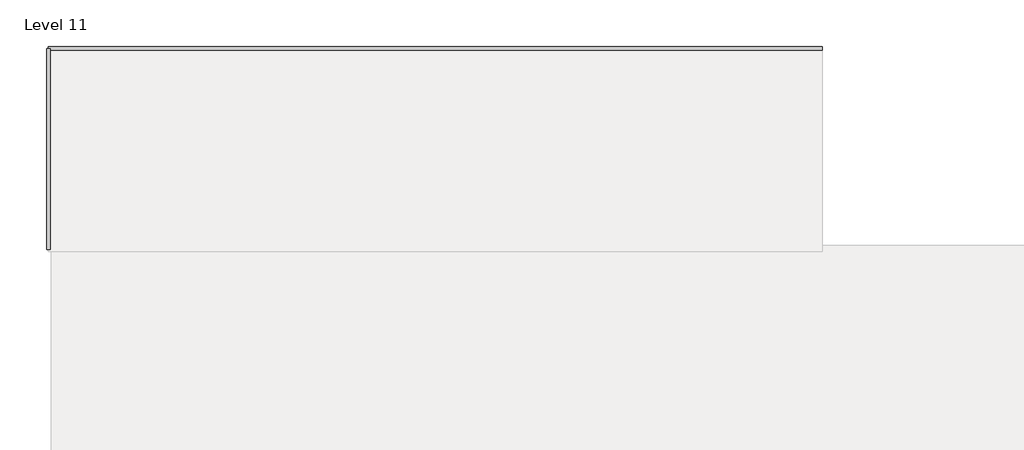
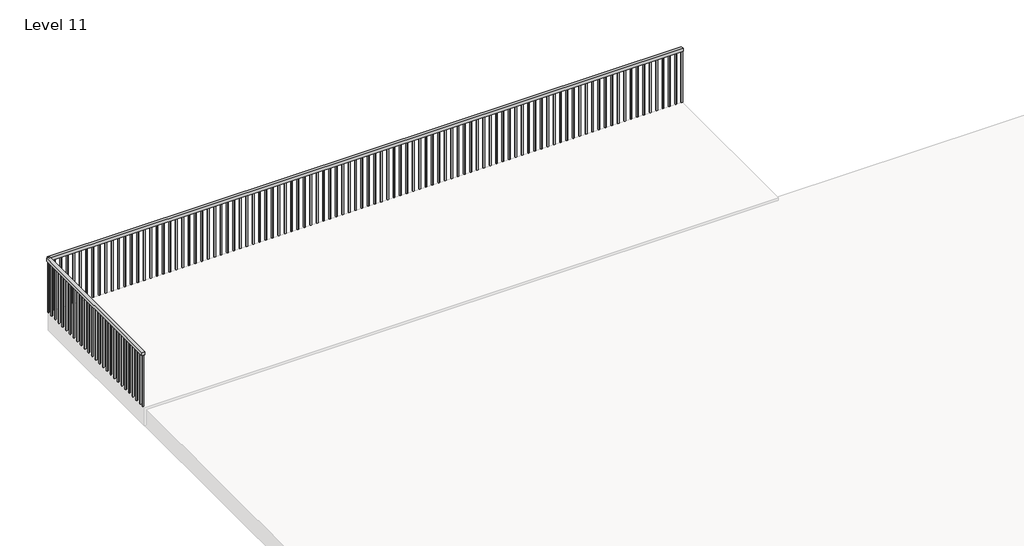
# One storey, part 3 of 5: 2 railings.
"""IFC4 building model written with IfcOpenShell, lengths in millimetres."""

from ifc_helpers import new_model, si_unit, frame, origin, place, context, project, spatial, polyline, outline, extrude, element, save

model = new_model("IFC4")

# Units and contexts
model_context = context("Model", 3, world=origin())
ifc_project = project(units=[si_unit("LENGTHUNIT", "METRE", prefix="MILLI")], contexts=[model_context])

# Site, building, storey
site = spatial("IfcSite", under=ifc_project)
building = spatial("IfcBuilding", under=site)
storey = spatial("IfcBuildingStorey", under=building, Name="Level 11", Elevation=15544.8)

# Railings
placement = place(None, origin())
element("IfcRailing", 1, ObjectType="Handrail - Rectangular", at=placement, inside=storey, context=model_context, shape_type="SweptSolid", body=[
    extrude(outline(polyline([(-13833.4638778, 17386.5959632), (-13833.4638778, 17437.3959632), (-3775.0638778, 17437.3959632), (-3775.0638778, 17386.5959632), (-13833.4638778, 17386.5959632)])), frame((0.0, 0.0, 16408.4), z_axis=(0.0, 0.0, 1.0), x_axis=(1.0, 0.0, 0.0)), (0.0, 0.0, 1.0), 50.8),
    extrude(outline(polyline([(-3886.1888778, 17402.4709632), (-3886.1888778, 17421.5209632), (-3867.1388778, 17421.5209632), (-3867.1388778, 17402.4709632), (-3886.1888778, 17402.4709632)])), frame((0.0, 0.0, 15544.8), z_axis=(0.0, 0.0, 1.0), x_axis=(1.0, 0.0, 0.0)), (0.0, 0.0, 1.0), 863.6),
    extrude(outline(polyline([(-3987.7888778, 17402.4709632), (-3987.7888778, 17421.5209632), (-3968.7388778, 17421.5209632), (-3968.7388778, 17402.4709632), (-3987.7888778, 17402.4709632)])), frame((0.0, 0.0, 15544.8), z_axis=(0.0, 0.0, 1.0), x_axis=(1.0, 0.0, 0.0)), (0.0, 0.0, 1.0), 863.6),
    extrude(outline(polyline([(-4089.3888778, 17402.4709632), (-4089.3888778, 17421.5209632), (-4070.3388778, 17421.5209632), (-4070.3388778, 17402.4709632), (-4089.3888778, 17402.4709632)])), frame((0.0, 0.0, 15544.8), z_axis=(0.0, 0.0, 1.0), x_axis=(1.0, 0.0, 0.0)), (0.0, 0.0, 1.0), 863.6),
    extrude(outline(polyline([(-4190.9888778, 17402.4709632), (-4190.9888778, 17421.5209632), (-4171.9388778, 17421.5209632), (-4171.9388778, 17402.4709632), (-4190.9888778, 17402.4709632)])), frame((0.0, 0.0, 15544.8), z_axis=(0.0, 0.0, 1.0), x_axis=(1.0, 0.0, 0.0)), (0.0, 0.0, 1.0), 863.6),
    extrude(outline(polyline([(-4292.5888778, 17402.4709632), (-4292.5888778, 17421.5209632), (-4273.5388778, 17421.5209632), (-4273.5388778, 17402.4709632), (-4292.5888778, 17402.4709632)])), frame((0.0, 0.0, 15544.8), z_axis=(0.0, 0.0, 1.0), x_axis=(1.0, 0.0, 0.0)), (0.0, 0.0, 1.0), 863.6),
    extrude(outline(polyline([(-4394.1888778, 17402.4709632), (-4394.1888778, 17421.5209632), (-4375.1388778, 17421.5209632), (-4375.1388778, 17402.4709632), (-4394.1888778, 17402.4709632)])), frame((0.0, 0.0, 15544.8), z_axis=(0.0, 0.0, 1.0), x_axis=(1.0, 0.0, 0.0)), (0.0, 0.0, 1.0), 863.6),
    extrude(outline(polyline([(-4495.7888778, 17402.4709632), (-4495.7888778, 17421.5209632), (-4476.7388778, 17421.5209632), (-4476.7388778, 17402.4709632), (-4495.7888778, 17402.4709632)])), frame((0.0, 0.0, 15544.8), z_axis=(0.0, 0.0, 1.0), x_axis=(1.0, 0.0, 0.0)), (0.0, 0.0, 1.0), 863.6),
    extrude(outline(polyline([(-4597.3888778, 17402.4709632), (-4597.3888778, 17421.5209632), (-4578.3388778, 17421.5209632), (-4578.3388778, 17402.4709632), (-4597.3888778, 17402.4709632)])), frame((0.0, 0.0, 15544.8), z_axis=(0.0, 0.0, 1.0), x_axis=(1.0, 0.0, 0.0)), (0.0, 0.0, 1.0), 863.6),
    extrude(outline(polyline([(-4698.9888778, 17402.4709632), (-4698.9888778, 17421.5209632), (-4679.9388778, 17421.5209632), (-4679.9388778, 17402.4709632), (-4698.9888778, 17402.4709632)])), frame((0.0, 0.0, 15544.8), z_axis=(0.0, 0.0, 1.0), x_axis=(1.0, 0.0, 0.0)), (0.0, 0.0, 1.0), 863.6),
    extrude(outline(polyline([(-4800.5888778, 17402.4709632), (-4800.5888778, 17421.5209632), (-4781.5388778, 17421.5209632), (-4781.5388778, 17402.4709632), (-4800.5888778, 17402.4709632)])), frame((0.0, 0.0, 15544.8), z_axis=(0.0, 0.0, 1.0), x_axis=(1.0, 0.0, 0.0)), (0.0, 0.0, 1.0), 863.6),
    extrude(outline(polyline([(-4902.1888778, 17402.4709632), (-4902.1888778, 17421.5209632), (-4883.1388778, 17421.5209632), (-4883.1388778, 17402.4709632), (-4902.1888778, 17402.4709632)])), frame((0.0, 0.0, 15544.8), z_axis=(0.0, 0.0, 1.0), x_axis=(1.0, 0.0, 0.0)), (0.0, 0.0, 1.0), 863.6),
    extrude(outline(polyline([(-5003.7888778, 17402.4709632), (-5003.7888778, 17421.5209632), (-4984.7388778, 17421.5209632), (-4984.7388778, 17402.4709632), (-5003.7888778, 17402.4709632)])), frame((0.0, 0.0, 15544.8), z_axis=(0.0, 0.0, 1.0), x_axis=(1.0, 0.0, 0.0)), (0.0, 0.0, 1.0), 863.6),
    extrude(outline(polyline([(-5105.3888778, 17402.4709632), (-5105.3888778, 17421.5209632), (-5086.3388778, 17421.5209632), (-5086.3388778, 17402.4709632), (-5105.3888778, 17402.4709632)])), frame((0.0, 0.0, 15544.8), z_axis=(0.0, 0.0, 1.0), x_axis=(1.0, 0.0, 0.0)), (0.0, 0.0, 1.0), 863.6),
    extrude(outline(polyline([(-5206.9888778, 17402.4709632), (-5206.9888778, 17421.5209632), (-5187.9388778, 17421.5209632), (-5187.9388778, 17402.4709632), (-5206.9888778, 17402.4709632)])), frame((0.0, 0.0, 15544.8), z_axis=(0.0, 0.0, 1.0), x_axis=(1.0, 0.0, 0.0)), (0.0, 0.0, 1.0), 863.6),
    extrude(outline(polyline([(-5308.5888778, 17402.4709632), (-5308.5888778, 17421.5209632), (-5289.5388778, 17421.5209632), (-5289.5388778, 17402.4709632), (-5308.5888778, 17402.4709632)])), frame((0.0, 0.0, 15544.8), z_axis=(0.0, 0.0, 1.0), x_axis=(1.0, 0.0, 0.0)), (0.0, 0.0, 1.0), 863.6),
    extrude(outline(polyline([(-5410.1888778, 17402.4709632), (-5410.1888778, 17421.5209632), (-5391.1388778, 17421.5209632), (-5391.1388778, 17402.4709632), (-5410.1888778, 17402.4709632)])), frame((0.0, 0.0, 15544.8), z_axis=(0.0, 0.0, 1.0), x_axis=(1.0, 0.0, 0.0)), (0.0, 0.0, 1.0), 863.6),
    extrude(outline(polyline([(-5511.7888778, 17402.4709632), (-5511.7888778, 17421.5209632), (-5492.7388778, 17421.5209632), (-5492.7388778, 17402.4709632), (-5511.7888778, 17402.4709632)])), frame((0.0, 0.0, 15544.8), z_axis=(0.0, 0.0, 1.0), x_axis=(1.0, 0.0, 0.0)), (0.0, 0.0, 1.0), 863.6),
    extrude(outline(polyline([(-5613.3888778, 17402.4709632), (-5613.3888778, 17421.5209632), (-5594.3388778, 17421.5209632), (-5594.3388778, 17402.4709632), (-5613.3888778, 17402.4709632)])), frame((0.0, 0.0, 15544.8), z_axis=(0.0, 0.0, 1.0), x_axis=(1.0, 0.0, 0.0)), (0.0, 0.0, 1.0), 863.6),
    extrude(outline(polyline([(-5714.9888778, 17402.4709632), (-5714.9888778, 17421.5209632), (-5695.9388778, 17421.5209632), (-5695.9388778, 17402.4709632), (-5714.9888778, 17402.4709632)])), frame((0.0, 0.0, 15544.8), z_axis=(0.0, 0.0, 1.0), x_axis=(1.0, 0.0, 0.0)), (0.0, 0.0, 1.0), 863.6),
    extrude(outline(polyline([(-5816.5888778, 17402.4709632), (-5816.5888778, 17421.5209632), (-5797.5388778, 17421.5209632), (-5797.5388778, 17402.4709632), (-5816.5888778, 17402.4709632)])), frame((0.0, 0.0, 15544.8), z_axis=(0.0, 0.0, 1.0), x_axis=(1.0, 0.0, 0.0)), (0.0, 0.0, 1.0), 863.6),
    extrude(outline(polyline([(-5918.1888778, 17402.4709632), (-5918.1888778, 17421.5209632), (-5899.1388778, 17421.5209632), (-5899.1388778, 17402.4709632), (-5918.1888778, 17402.4709632)])), frame((0.0, 0.0, 15544.8), z_axis=(0.0, 0.0, 1.0), x_axis=(1.0, 0.0, 0.0)), (0.0, 0.0, 1.0), 863.6),
    extrude(outline(polyline([(-6019.7888778, 17402.4709632), (-6019.7888778, 17421.5209632), (-6000.7388778, 17421.5209632), (-6000.7388778, 17402.4709632), (-6019.7888778, 17402.4709632)])), frame((0.0, 0.0, 15544.8), z_axis=(0.0, 0.0, 1.0), x_axis=(1.0, 0.0, 0.0)), (0.0, 0.0, 1.0), 863.6),
    extrude(outline(polyline([(-6121.3888778, 17402.4709632), (-6121.3888778, 17421.5209632), (-6102.3388778, 17421.5209632), (-6102.3388778, 17402.4709632), (-6121.3888778, 17402.4709632)])), frame((0.0, 0.0, 15544.8), z_axis=(0.0, 0.0, 1.0), x_axis=(1.0, 0.0, 0.0)), (0.0, 0.0, 1.0), 863.6),
    extrude(outline(polyline([(-6222.9888778, 17402.4709632), (-6222.9888778, 17421.5209632), (-6203.9388778, 17421.5209632), (-6203.9388778, 17402.4709632), (-6222.9888778, 17402.4709632)])), frame((0.0, 0.0, 15544.8), z_axis=(0.0, 0.0, 1.0), x_axis=(1.0, 0.0, 0.0)), (0.0, 0.0, 1.0), 863.6),
    extrude(outline(polyline([(-6324.5888778, 17402.4709632), (-6324.5888778, 17421.5209632), (-6305.5388778, 17421.5209632), (-6305.5388778, 17402.4709632), (-6324.5888778, 17402.4709632)])), frame((0.0, 0.0, 15544.8), z_axis=(0.0, 0.0, 1.0), x_axis=(1.0, 0.0, 0.0)), (0.0, 0.0, 1.0), 863.6),
    extrude(outline(polyline([(-6426.1888778, 17402.4709632), (-6426.1888778, 17421.5209632), (-6407.1388778, 17421.5209632), (-6407.1388778, 17402.4709632), (-6426.1888778, 17402.4709632)])), frame((0.0, 0.0, 15544.8), z_axis=(0.0, 0.0, 1.0), x_axis=(1.0, 0.0, 0.0)), (0.0, 0.0, 1.0), 863.6),
    extrude(outline(polyline([(-6527.7888778, 17402.4709632), (-6527.7888778, 17421.5209632), (-6508.7388778, 17421.5209632), (-6508.7388778, 17402.4709632), (-6527.7888778, 17402.4709632)])), frame((0.0, 0.0, 15544.8), z_axis=(0.0, 0.0, 1.0), x_axis=(1.0, 0.0, 0.0)), (0.0, 0.0, 1.0), 863.6),
    extrude(outline(polyline([(-6629.3888778, 17402.4709632), (-6629.3888778, 17421.5209632), (-6610.3388778, 17421.5209632), (-6610.3388778, 17402.4709632), (-6629.3888778, 17402.4709632)])), frame((0.0, 0.0, 15544.8), z_axis=(0.0, 0.0, 1.0), x_axis=(1.0, 0.0, 0.0)), (0.0, 0.0, 1.0), 863.6),
    extrude(outline(polyline([(-6730.9888778, 17402.4709632), (-6730.9888778, 17421.5209632), (-6711.9388778, 17421.5209632), (-6711.9388778, 17402.4709632), (-6730.9888778, 17402.4709632)])), frame((0.0, 0.0, 15544.8), z_axis=(0.0, 0.0, 1.0), x_axis=(1.0, 0.0, 0.0)), (0.0, 0.0, 1.0), 863.6),
    extrude(outline(polyline([(-6832.5888778, 17402.4709632), (-6832.5888778, 17421.5209632), (-6813.5388778, 17421.5209632), (-6813.5388778, 17402.4709632), (-6832.5888778, 17402.4709632)])), frame((0.0, 0.0, 15544.8), z_axis=(0.0, 0.0, 1.0), x_axis=(1.0, 0.0, 0.0)), (0.0, 0.0, 1.0), 863.6),
    extrude(outline(polyline([(-6934.1888778, 17402.4709632), (-6934.1888778, 17421.5209632), (-6915.1388778, 17421.5209632), (-6915.1388778, 17402.4709632), (-6934.1888778, 17402.4709632)])), frame((0.0, 0.0, 15544.8), z_axis=(0.0, 0.0, 1.0), x_axis=(1.0, 0.0, 0.0)), (0.0, 0.0, 1.0), 863.6),
    extrude(outline(polyline([(-7035.7888778, 17402.4709632), (-7035.7888778, 17421.5209632), (-7016.7388778, 17421.5209632), (-7016.7388778, 17402.4709632), (-7035.7888778, 17402.4709632)])), frame((0.0, 0.0, 15544.8), z_axis=(0.0, 0.0, 1.0), x_axis=(1.0, 0.0, 0.0)), (0.0, 0.0, 1.0), 863.6),
    extrude(outline(polyline([(-7137.3888778, 17402.4709632), (-7137.3888778, 17421.5209632), (-7118.3388778, 17421.5209632), (-7118.3388778, 17402.4709632), (-7137.3888778, 17402.4709632)])), frame((0.0, 0.0, 15544.8), z_axis=(0.0, 0.0, 1.0), x_axis=(1.0, 0.0, 0.0)), (0.0, 0.0, 1.0), 863.6),
    extrude(outline(polyline([(-7238.9888778, 17402.4709632), (-7238.9888778, 17421.5209632), (-7219.9388778, 17421.5209632), (-7219.9388778, 17402.4709632), (-7238.9888778, 17402.4709632)])), frame((0.0, 0.0, 15544.8), z_axis=(0.0, 0.0, 1.0), x_axis=(1.0, 0.0, 0.0)), (0.0, 0.0, 1.0), 863.6),
    extrude(outline(polyline([(-7340.5888778, 17402.4709632), (-7340.5888778, 17421.5209632), (-7321.5388778, 17421.5209632), (-7321.5388778, 17402.4709632), (-7340.5888778, 17402.4709632)])), frame((0.0, 0.0, 15544.8), z_axis=(0.0, 0.0, 1.0), x_axis=(1.0, 0.0, 0.0)), (0.0, 0.0, 1.0), 863.6),
    extrude(outline(polyline([(-7442.1888778, 17402.4709632), (-7442.1888778, 17421.5209632), (-7423.1388778, 17421.5209632), (-7423.1388778, 17402.4709632), (-7442.1888778, 17402.4709632)])), frame((0.0, 0.0, 15544.8), z_axis=(0.0, 0.0, 1.0), x_axis=(1.0, 0.0, 0.0)), (0.0, 0.0, 1.0), 863.6),
    extrude(outline(polyline([(-7543.7888778, 17402.4709632), (-7543.7888778, 17421.5209632), (-7524.7388778, 17421.5209632), (-7524.7388778, 17402.4709632), (-7543.7888778, 17402.4709632)])), frame((0.0, 0.0, 15544.8), z_axis=(0.0, 0.0, 1.0), x_axis=(1.0, 0.0, 0.0)), (0.0, 0.0, 1.0), 863.6),
    extrude(outline(polyline([(-7645.3888778, 17402.4709632), (-7645.3888778, 17421.5209632), (-7626.3388778, 17421.5209632), (-7626.3388778, 17402.4709632), (-7645.3888778, 17402.4709632)])), frame((0.0, 0.0, 15544.8), z_axis=(0.0, 0.0, 1.0), x_axis=(1.0, 0.0, 0.0)), (0.0, 0.0, 1.0), 863.6),
    extrude(outline(polyline([(-7746.9888778, 17402.4709632), (-7746.9888778, 17421.5209632), (-7727.9388778, 17421.5209632), (-7727.9388778, 17402.4709632), (-7746.9888778, 17402.4709632)])), frame((0.0, 0.0, 15544.8), z_axis=(0.0, 0.0, 1.0), x_axis=(1.0, 0.0, 0.0)), (0.0, 0.0, 1.0), 863.6),
    extrude(outline(polyline([(-7848.5888778, 17402.4709632), (-7848.5888778, 17421.5209632), (-7829.5388778, 17421.5209632), (-7829.5388778, 17402.4709632), (-7848.5888778, 17402.4709632)])), frame((0.0, 0.0, 15544.8), z_axis=(0.0, 0.0, 1.0), x_axis=(1.0, 0.0, 0.0)), (0.0, 0.0, 1.0), 863.6),
    extrude(outline(polyline([(-7950.1888778, 17402.4709632), (-7950.1888778, 17421.5209632), (-7931.1388778, 17421.5209632), (-7931.1388778, 17402.4709632), (-7950.1888778, 17402.4709632)])), frame((0.0, 0.0, 15544.8), z_axis=(0.0, 0.0, 1.0), x_axis=(1.0, 0.0, 0.0)), (0.0, 0.0, 1.0), 863.6),
    extrude(outline(polyline([(-8051.7888778, 17402.4709632), (-8051.7888778, 17421.5209632), (-8032.7388778, 17421.5209632), (-8032.7388778, 17402.4709632), (-8051.7888778, 17402.4709632)])), frame((0.0, 0.0, 15544.8), z_axis=(0.0, 0.0, 1.0), x_axis=(1.0, 0.0, 0.0)), (0.0, 0.0, 1.0), 863.6),
    extrude(outline(polyline([(-8153.3888778, 17402.4709632), (-8153.3888778, 17421.5209632), (-8134.3388778, 17421.5209632), (-8134.3388778, 17402.4709632), (-8153.3888778, 17402.4709632)])), frame((0.0, 0.0, 15544.8), z_axis=(0.0, 0.0, 1.0), x_axis=(1.0, 0.0, 0.0)), (0.0, 0.0, 1.0), 863.6),
    extrude(outline(polyline([(-8254.9888778, 17402.4709632), (-8254.9888778, 17421.5209632), (-8235.9388778, 17421.5209632), (-8235.9388778, 17402.4709632), (-8254.9888778, 17402.4709632)])), frame((0.0, 0.0, 15544.8), z_axis=(0.0, 0.0, 1.0), x_axis=(1.0, 0.0, 0.0)), (0.0, 0.0, 1.0), 863.6),
    extrude(outline(polyline([(-8356.5888778, 17402.4709632), (-8356.5888778, 17421.5209632), (-8337.5388778, 17421.5209632), (-8337.5388778, 17402.4709632), (-8356.5888778, 17402.4709632)])), frame((0.0, 0.0, 15544.8), z_axis=(0.0, 0.0, 1.0), x_axis=(1.0, 0.0, 0.0)), (0.0, 0.0, 1.0), 863.6),
    extrude(outline(polyline([(-8458.1888778, 17402.4709632), (-8458.1888778, 17421.5209632), (-8439.1388778, 17421.5209632), (-8439.1388778, 17402.4709632), (-8458.1888778, 17402.4709632)])), frame((0.0, 0.0, 15544.8), z_axis=(0.0, 0.0, 1.0), x_axis=(1.0, 0.0, 0.0)), (0.0, 0.0, 1.0), 863.6),
    extrude(outline(polyline([(-8559.7888778, 17402.4709632), (-8559.7888778, 17421.5209632), (-8540.7388778, 17421.5209632), (-8540.7388778, 17402.4709632), (-8559.7888778, 17402.4709632)])), frame((0.0, 0.0, 15544.8), z_axis=(0.0, 0.0, 1.0), x_axis=(1.0, 0.0, 0.0)), (0.0, 0.0, 1.0), 863.6),
    extrude(outline(polyline([(-8661.3888778, 17402.4709632), (-8661.3888778, 17421.5209632), (-8642.3388778, 17421.5209632), (-8642.3388778, 17402.4709632), (-8661.3888778, 17402.4709632)])), frame((0.0, 0.0, 15544.8), z_axis=(0.0, 0.0, 1.0), x_axis=(1.0, 0.0, 0.0)), (0.0, 0.0, 1.0), 863.6),
    extrude(outline(polyline([(-8762.9888778, 17402.4709632), (-8762.9888778, 17421.5209632), (-8743.9388778, 17421.5209632), (-8743.9388778, 17402.4709632), (-8762.9888778, 17402.4709632)])), frame((0.0, 0.0, 15544.8), z_axis=(0.0, 0.0, 1.0), x_axis=(1.0, 0.0, 0.0)), (0.0, 0.0, 1.0), 863.6),
    extrude(outline(polyline([(-8864.5888778, 17402.4709632), (-8864.5888778, 17421.5209632), (-8845.5388778, 17421.5209632), (-8845.5388778, 17402.4709632), (-8864.5888778, 17402.4709632)])), frame((0.0, 0.0, 15544.8), z_axis=(0.0, 0.0, 1.0), x_axis=(1.0, 0.0, 0.0)), (0.0, 0.0, 1.0), 863.6),
    extrude(outline(polyline([(-8966.1888778, 17402.4709632), (-8966.1888778, 17421.5209632), (-8947.1388778, 17421.5209632), (-8947.1388778, 17402.4709632), (-8966.1888778, 17402.4709632)])), frame((0.0, 0.0, 15544.8), z_axis=(0.0, 0.0, 1.0), x_axis=(1.0, 0.0, 0.0)), (0.0, 0.0, 1.0), 863.6),
    extrude(outline(polyline([(-9067.7888778, 17402.4709632), (-9067.7888778, 17421.5209632), (-9048.7388778, 17421.5209632), (-9048.7388778, 17402.4709632), (-9067.7888778, 17402.4709632)])), frame((0.0, 0.0, 15544.8), z_axis=(0.0, 0.0, 1.0), x_axis=(1.0, 0.0, 0.0)), (0.0, 0.0, 1.0), 863.6),
    extrude(outline(polyline([(-9169.3888778, 17402.4709632), (-9169.3888778, 17421.5209632), (-9150.3388778, 17421.5209632), (-9150.3388778, 17402.4709632), (-9169.3888778, 17402.4709632)])), frame((0.0, 0.0, 15544.8), z_axis=(0.0, 0.0, 1.0), x_axis=(1.0, 0.0, 0.0)), (0.0, 0.0, 1.0), 863.6),
    extrude(outline(polyline([(-9270.9888778, 17402.4709632), (-9270.9888778, 17421.5209632), (-9251.9388778, 17421.5209632), (-9251.9388778, 17402.4709632), (-9270.9888778, 17402.4709632)])), frame((0.0, 0.0, 15544.8), z_axis=(0.0, 0.0, 1.0), x_axis=(1.0, 0.0, 0.0)), (0.0, 0.0, 1.0), 863.6),
    extrude(outline(polyline([(-9372.5888778, 17402.4709632), (-9372.5888778, 17421.5209632), (-9353.5388778, 17421.5209632), (-9353.5388778, 17402.4709632), (-9372.5888778, 17402.4709632)])), frame((0.0, 0.0, 15544.8), z_axis=(0.0, 0.0, 1.0), x_axis=(1.0, 0.0, 0.0)), (0.0, 0.0, 1.0), 863.6),
    extrude(outline(polyline([(-9474.1888778, 17402.4709632), (-9474.1888778, 17421.5209632), (-9455.1388778, 17421.5209632), (-9455.1388778, 17402.4709632), (-9474.1888778, 17402.4709632)])), frame((0.0, 0.0, 15544.8), z_axis=(0.0, 0.0, 1.0), x_axis=(1.0, 0.0, 0.0)), (0.0, 0.0, 1.0), 863.6),
    extrude(outline(polyline([(-9575.7888778, 17402.4709632), (-9575.7888778, 17421.5209632), (-9556.7388778, 17421.5209632), (-9556.7388778, 17402.4709632), (-9575.7888778, 17402.4709632)])), frame((0.0, 0.0, 15544.8), z_axis=(0.0, 0.0, 1.0), x_axis=(1.0, 0.0, 0.0)), (0.0, 0.0, 1.0), 863.6),
    extrude(outline(polyline([(-9677.3888778, 17402.4709632), (-9677.3888778, 17421.5209632), (-9658.3388778, 17421.5209632), (-9658.3388778, 17402.4709632), (-9677.3888778, 17402.4709632)])), frame((0.0, 0.0, 15544.8), z_axis=(0.0, 0.0, 1.0), x_axis=(1.0, 0.0, 0.0)), (0.0, 0.0, 1.0), 863.6),
    extrude(outline(polyline([(-9778.9888778, 17402.4709632), (-9778.9888778, 17421.5209632), (-9759.9388778, 17421.5209632), (-9759.9388778, 17402.4709632), (-9778.9888778, 17402.4709632)])), frame((0.0, 0.0, 15544.8), z_axis=(0.0, 0.0, 1.0), x_axis=(1.0, 0.0, 0.0)), (0.0, 0.0, 1.0), 863.6),
    extrude(outline(polyline([(-9880.5888778, 17402.4709632), (-9880.5888778, 17421.5209632), (-9861.5388778, 17421.5209632), (-9861.5388778, 17402.4709632), (-9880.5888778, 17402.4709632)])), frame((0.0, 0.0, 15544.8), z_axis=(0.0, 0.0, 1.0), x_axis=(1.0, 0.0, 0.0)), (0.0, 0.0, 1.0), 863.6),
    extrude(outline(polyline([(-9982.1888778, 17402.4709632), (-9982.1888778, 17421.5209632), (-9963.1388778, 17421.5209632), (-9963.1388778, 17402.4709632), (-9982.1888778, 17402.4709632)])), frame((0.0, 0.0, 15544.8), z_axis=(0.0, 0.0, 1.0), x_axis=(1.0, 0.0, 0.0)), (0.0, 0.0, 1.0), 863.6),
    extrude(outline(polyline([(-10083.7888778, 17402.4709632), (-10083.7888778, 17421.5209632), (-10064.7388778, 17421.5209632), (-10064.7388778, 17402.4709632), (-10083.7888778, 17402.4709632)])), frame((0.0, 0.0, 15544.8), z_axis=(0.0, 0.0, 1.0), x_axis=(1.0, 0.0, 0.0)), (0.0, 0.0, 1.0), 863.6),
    extrude(outline(polyline([(-10185.3888778, 17402.4709632), (-10185.3888778, 17421.5209632), (-10166.3388778, 17421.5209632), (-10166.3388778, 17402.4709632), (-10185.3888778, 17402.4709632)])), frame((0.0, 0.0, 15544.8), z_axis=(0.0, 0.0, 1.0), x_axis=(1.0, 0.0, 0.0)), (0.0, 0.0, 1.0), 863.6),
    extrude(outline(polyline([(-10286.9888778, 17402.4709632), (-10286.9888778, 17421.5209632), (-10267.9388778, 17421.5209632), (-10267.9388778, 17402.4709632), (-10286.9888778, 17402.4709632)])), frame((0.0, 0.0, 15544.8), z_axis=(0.0, 0.0, 1.0), x_axis=(1.0, 0.0, 0.0)), (0.0, 0.0, 1.0), 863.6),
    extrude(outline(polyline([(-10388.5888778, 17402.4709632), (-10388.5888778, 17421.5209632), (-10369.5388778, 17421.5209632), (-10369.5388778, 17402.4709632), (-10388.5888778, 17402.4709632)])), frame((0.0, 0.0, 15544.8), z_axis=(0.0, 0.0, 1.0), x_axis=(1.0, 0.0, 0.0)), (0.0, 0.0, 1.0), 863.6),
    extrude(outline(polyline([(-10490.1888778, 17402.4709632), (-10490.1888778, 17421.5209632), (-10471.1388778, 17421.5209632), (-10471.1388778, 17402.4709632), (-10490.1888778, 17402.4709632)])), frame((0.0, 0.0, 15544.8), z_axis=(0.0, 0.0, 1.0), x_axis=(1.0, 0.0, 0.0)), (0.0, 0.0, 1.0), 863.6),
    extrude(outline(polyline([(-10591.7888778, 17402.4709632), (-10591.7888778, 17421.5209632), (-10572.7388778, 17421.5209632), (-10572.7388778, 17402.4709632), (-10591.7888778, 17402.4709632)])), frame((0.0, 0.0, 15544.8), z_axis=(0.0, 0.0, 1.0), x_axis=(1.0, 0.0, 0.0)), (0.0, 0.0, 1.0), 863.6),
    extrude(outline(polyline([(-10693.3888778, 17402.4709632), (-10693.3888778, 17421.5209632), (-10674.3388778, 17421.5209632), (-10674.3388778, 17402.4709632), (-10693.3888778, 17402.4709632)])), frame((0.0, 0.0, 15544.8), z_axis=(0.0, 0.0, 1.0), x_axis=(1.0, 0.0, 0.0)), (0.0, 0.0, 1.0), 863.6),
    extrude(outline(polyline([(-10794.9888778, 17402.4709632), (-10794.9888778, 17421.5209632), (-10775.9388778, 17421.5209632), (-10775.9388778, 17402.4709632), (-10794.9888778, 17402.4709632)])), frame((0.0, 0.0, 15544.8), z_axis=(0.0, 0.0, 1.0), x_axis=(1.0, 0.0, 0.0)), (0.0, 0.0, 1.0), 863.6),
    extrude(outline(polyline([(-10896.5888778, 17402.4709632), (-10896.5888778, 17421.5209632), (-10877.5388778, 17421.5209632), (-10877.5388778, 17402.4709632), (-10896.5888778, 17402.4709632)])), frame((0.0, 0.0, 15544.8), z_axis=(0.0, 0.0, 1.0), x_axis=(1.0, 0.0, 0.0)), (0.0, 0.0, 1.0), 863.6),
    extrude(outline(polyline([(-10998.1888778, 17402.4709632), (-10998.1888778, 17421.5209632), (-10979.1388778, 17421.5209632), (-10979.1388778, 17402.4709632), (-10998.1888778, 17402.4709632)])), frame((0.0, 0.0, 15544.8), z_axis=(0.0, 0.0, 1.0), x_axis=(1.0, 0.0, 0.0)), (0.0, 0.0, 1.0), 863.6),
    extrude(outline(polyline([(-11099.7888778, 17402.4709632), (-11099.7888778, 17421.5209632), (-11080.7388778, 17421.5209632), (-11080.7388778, 17402.4709632), (-11099.7888778, 17402.4709632)])), frame((0.0, 0.0, 15544.8), z_axis=(0.0, 0.0, 1.0), x_axis=(1.0, 0.0, 0.0)), (0.0, 0.0, 1.0), 863.6),
    extrude(outline(polyline([(-11201.3888778, 17402.4709632), (-11201.3888778, 17421.5209632), (-11182.3388778, 17421.5209632), (-11182.3388778, 17402.4709632), (-11201.3888778, 17402.4709632)])), frame((0.0, 0.0, 15544.8), z_axis=(0.0, 0.0, 1.0), x_axis=(1.0, 0.0, 0.0)), (0.0, 0.0, 1.0), 863.6),
    extrude(outline(polyline([(-11302.9888778, 17402.4709632), (-11302.9888778, 17421.5209632), (-11283.9388778, 17421.5209632), (-11283.9388778, 17402.4709632), (-11302.9888778, 17402.4709632)])), frame((0.0, 0.0, 15544.8), z_axis=(0.0, 0.0, 1.0), x_axis=(1.0, 0.0, 0.0)), (0.0, 0.0, 1.0), 863.6),
    extrude(outline(polyline([(-11404.5888778, 17402.4709632), (-11404.5888778, 17421.5209632), (-11385.5388778, 17421.5209632), (-11385.5388778, 17402.4709632), (-11404.5888778, 17402.4709632)])), frame((0.0, 0.0, 15544.8), z_axis=(0.0, 0.0, 1.0), x_axis=(1.0, 0.0, 0.0)), (0.0, 0.0, 1.0), 863.6),
    extrude(outline(polyline([(-11506.1888778, 17402.4709632), (-11506.1888778, 17421.5209632), (-11487.1388778, 17421.5209632), (-11487.1388778, 17402.4709632), (-11506.1888778, 17402.4709632)])), frame((0.0, 0.0, 15544.8), z_axis=(0.0, 0.0, 1.0), x_axis=(1.0, 0.0, 0.0)), (0.0, 0.0, 1.0), 863.6),
    extrude(outline(polyline([(-11607.7888778, 17402.4709632), (-11607.7888778, 17421.5209632), (-11588.7388778, 17421.5209632), (-11588.7388778, 17402.4709632), (-11607.7888778, 17402.4709632)])), frame((0.0, 0.0, 15544.8), z_axis=(0.0, 0.0, 1.0), x_axis=(1.0, 0.0, 0.0)), (0.0, 0.0, 1.0), 863.6),
    extrude(outline(polyline([(-11709.3888778, 17402.4709632), (-11709.3888778, 17421.5209632), (-11690.3388778, 17421.5209632), (-11690.3388778, 17402.4709632), (-11709.3888778, 17402.4709632)])), frame((0.0, 0.0, 15544.8), z_axis=(0.0, 0.0, 1.0), x_axis=(1.0, 0.0, 0.0)), (0.0, 0.0, 1.0), 863.6),
    extrude(outline(polyline([(-11810.9888778, 17402.4709632), (-11810.9888778, 17421.5209632), (-11791.9388778, 17421.5209632), (-11791.9388778, 17402.4709632), (-11810.9888778, 17402.4709632)])), frame((0.0, 0.0, 15544.8), z_axis=(0.0, 0.0, 1.0), x_axis=(1.0, 0.0, 0.0)), (0.0, 0.0, 1.0), 863.6),
    extrude(outline(polyline([(-11912.5888778, 17402.4709632), (-11912.5888778, 17421.5209632), (-11893.5388778, 17421.5209632), (-11893.5388778, 17402.4709632), (-11912.5888778, 17402.4709632)])), frame((0.0, 0.0, 15544.8), z_axis=(0.0, 0.0, 1.0), x_axis=(1.0, 0.0, 0.0)), (0.0, 0.0, 1.0), 863.6),
    extrude(outline(polyline([(-12014.1888778, 17402.4709632), (-12014.1888778, 17421.5209632), (-11995.1388778, 17421.5209632), (-11995.1388778, 17402.4709632), (-12014.1888778, 17402.4709632)])), frame((0.0, 0.0, 15544.8), z_axis=(0.0, 0.0, 1.0), x_axis=(1.0, 0.0, 0.0)), (0.0, 0.0, 1.0), 863.6),
    extrude(outline(polyline([(-12115.7888778, 17402.4709632), (-12115.7888778, 17421.5209632), (-12096.7388778, 17421.5209632), (-12096.7388778, 17402.4709632), (-12115.7888778, 17402.4709632)])), frame((0.0, 0.0, 15544.8), z_axis=(0.0, 0.0, 1.0), x_axis=(1.0, 0.0, 0.0)), (0.0, 0.0, 1.0), 863.6),
    extrude(outline(polyline([(-12217.3888778, 17402.4709632), (-12217.3888778, 17421.5209632), (-12198.3388778, 17421.5209632), (-12198.3388778, 17402.4709632), (-12217.3888778, 17402.4709632)])), frame((0.0, 0.0, 15544.8), z_axis=(0.0, 0.0, 1.0), x_axis=(1.0, 0.0, 0.0)), (0.0, 0.0, 1.0), 863.6),
    extrude(outline(polyline([(-12318.9888778, 17402.4709632), (-12318.9888778, 17421.5209632), (-12299.9388778, 17421.5209632), (-12299.9388778, 17402.4709632), (-12318.9888778, 17402.4709632)])), frame((0.0, 0.0, 15544.8), z_axis=(0.0, 0.0, 1.0), x_axis=(1.0, 0.0, 0.0)), (0.0, 0.0, 1.0), 863.6),
    extrude(outline(polyline([(-12420.5888778, 17402.4709632), (-12420.5888778, 17421.5209632), (-12401.5388778, 17421.5209632), (-12401.5388778, 17402.4709632), (-12420.5888778, 17402.4709632)])), frame((0.0, 0.0, 15544.8), z_axis=(0.0, 0.0, 1.0), x_axis=(1.0, 0.0, 0.0)), (0.0, 0.0, 1.0), 863.6),
    extrude(outline(polyline([(-12522.1888778, 17402.4709632), (-12522.1888778, 17421.5209632), (-12503.1388778, 17421.5209632), (-12503.1388778, 17402.4709632), (-12522.1888778, 17402.4709632)])), frame((0.0, 0.0, 15544.8), z_axis=(0.0, 0.0, 1.0), x_axis=(1.0, 0.0, 0.0)), (0.0, 0.0, 1.0), 863.6),
    extrude(outline(polyline([(-12623.7888778, 17402.4709632), (-12623.7888778, 17421.5209632), (-12604.7388778, 17421.5209632), (-12604.7388778, 17402.4709632), (-12623.7888778, 17402.4709632)])), frame((0.0, 0.0, 15544.8), z_axis=(0.0, 0.0, 1.0), x_axis=(1.0, 0.0, 0.0)), (0.0, 0.0, 1.0), 863.6),
    extrude(outline(polyline([(-12725.3888778, 17402.4709632), (-12725.3888778, 17421.5209632), (-12706.3388778, 17421.5209632), (-12706.3388778, 17402.4709632), (-12725.3888778, 17402.4709632)])), frame((0.0, 0.0, 15544.8), z_axis=(0.0, 0.0, 1.0), x_axis=(1.0, 0.0, 0.0)), (0.0, 0.0, 1.0), 863.6),
    extrude(outline(polyline([(-12826.9888778, 17402.4709632), (-12826.9888778, 17421.5209632), (-12807.9388778, 17421.5209632), (-12807.9388778, 17402.4709632), (-12826.9888778, 17402.4709632)])), frame((0.0, 0.0, 15544.8), z_axis=(0.0, 0.0, 1.0), x_axis=(1.0, 0.0, 0.0)), (0.0, 0.0, 1.0), 863.6),
    extrude(outline(polyline([(-12928.5888778, 17402.4709632), (-12928.5888778, 17421.5209632), (-12909.5388778, 17421.5209632), (-12909.5388778, 17402.4709632), (-12928.5888778, 17402.4709632)])), frame((0.0, 0.0, 15544.8), z_axis=(0.0, 0.0, 1.0), x_axis=(1.0, 0.0, 0.0)), (0.0, 0.0, 1.0), 863.6),
    extrude(outline(polyline([(-13030.1888778, 17402.4709632), (-13030.1888778, 17421.5209632), (-13011.1388778, 17421.5209632), (-13011.1388778, 17402.4709632), (-13030.1888778, 17402.4709632)])), frame((0.0, 0.0, 15544.8), z_axis=(0.0, 0.0, 1.0), x_axis=(1.0, 0.0, 0.0)), (0.0, 0.0, 1.0), 863.6),
    extrude(outline(polyline([(-13131.7888778, 17402.4709632), (-13131.7888778, 17421.5209632), (-13112.7388778, 17421.5209632), (-13112.7388778, 17402.4709632), (-13131.7888778, 17402.4709632)])), frame((0.0, 0.0, 15544.8), z_axis=(0.0, 0.0, 1.0), x_axis=(1.0, 0.0, 0.0)), (0.0, 0.0, 1.0), 863.6),
    extrude(outline(polyline([(-13233.3888778, 17402.4709632), (-13233.3888778, 17421.5209632), (-13214.3388778, 17421.5209632), (-13214.3388778, 17402.4709632), (-13233.3888778, 17402.4709632)])), frame((0.0, 0.0, 15544.8), z_axis=(0.0, 0.0, 1.0), x_axis=(1.0, 0.0, 0.0)), (0.0, 0.0, 1.0), 863.6),
    extrude(outline(polyline([(-13334.9888778, 17402.4709632), (-13334.9888778, 17421.5209632), (-13315.9388778, 17421.5209632), (-13315.9388778, 17402.4709632), (-13334.9888778, 17402.4709632)])), frame((0.0, 0.0, 15544.8), z_axis=(0.0, 0.0, 1.0), x_axis=(1.0, 0.0, 0.0)), (0.0, 0.0, 1.0), 863.6),
    extrude(outline(polyline([(-13436.5888778, 17402.4709632), (-13436.5888778, 17421.5209632), (-13417.5388778, 17421.5209632), (-13417.5388778, 17402.4709632), (-13436.5888778, 17402.4709632)])), frame((0.0, 0.0, 15544.8), z_axis=(0.0, 0.0, 1.0), x_axis=(1.0, 0.0, 0.0)), (0.0, 0.0, 1.0), 863.6),
    extrude(outline(polyline([(-13538.1888778, 17402.4709632), (-13538.1888778, 17421.5209632), (-13519.1388778, 17421.5209632), (-13519.1388778, 17402.4709632), (-13538.1888778, 17402.4709632)])), frame((0.0, 0.0, 15544.8), z_axis=(0.0, 0.0, 1.0), x_axis=(1.0, 0.0, 0.0)), (0.0, 0.0, 1.0), 863.6),
    extrude(outline(polyline([(-13639.7888778, 17402.4709632), (-13639.7888778, 17421.5209632), (-13620.7388778, 17421.5209632), (-13620.7388778, 17402.4709632), (-13639.7888778, 17402.4709632)])), frame((0.0, 0.0, 15544.8), z_axis=(0.0, 0.0, 1.0), x_axis=(1.0, 0.0, 0.0)), (0.0, 0.0, 1.0), 863.6),
    extrude(outline(polyline([(-13741.3888778, 17402.4709632), (-13741.3888778, 17421.5209632), (-13722.3388778, 17421.5209632), (-13722.3388778, 17402.4709632), (-13741.3888778, 17402.4709632)])), frame((0.0, 0.0, 15544.8), z_axis=(0.0, 0.0, 1.0), x_axis=(1.0, 0.0, 0.0)), (0.0, 0.0, 1.0), 863.6),
    extrude(outline(polyline([(-3794.1138778, 17402.4709632), (-3794.1138778, 17421.5209632), (-3775.0638778, 17421.5209632), (-3775.0638778, 17402.4709632), (-3794.1138778, 17402.4709632)])), frame((0.0, 0.0, 15544.8), z_axis=(0.0, 0.0, 1.0), x_axis=(1.0, 0.0, 0.0)), (0.0, 0.0, 1.0), 863.6),
    extrude(outline(polyline([(-13833.4638778, 17402.4709632), (-13833.4638778, 17421.5209632), (-13814.4138778, 17421.5209632), (-13814.4138778, 17402.4709632), (-13833.4638778, 17402.4709632)])), frame((0.0, 0.0, 15544.8), z_axis=(0.0, 0.0, 1.0), x_axis=(1.0, 0.0, 0.0)), (0.0, 0.0, 1.0), 863.6),
])
element("IfcRailing", 2, ObjectType="Handrail - Rectangular", at=placement, inside=storey, context=model_context, shape_type="SweptSolid", body=[
    extrude(outline(polyline([(-13858.8638778, 17410.2237525), (-13808.0638778, 17410.2237525), (-13808.0638778, 14794.0237525), (-13858.8638778, 14794.0237525), (-13858.8638778, 17410.2237525)])), frame((0.0, 0.0, 16408.4), z_axis=(0.0, 0.0, 1.0), x_axis=(1.0, 0.0, 0.0)), (0.0, 0.0, 1.0), 50.8),
    extrude(outline(polyline([(-13842.9888778, 14879.7487525), (-13823.9388778, 14879.7487525), (-13823.9388778, 14860.6987525), (-13842.9888778, 14860.6987525), (-13842.9888778, 14879.7487525)])), frame((0.0, 0.0, 15544.8), z_axis=(0.0, 0.0, 1.0), x_axis=(1.0, 0.0, 0.0)), (0.0, 0.0, 1.0), 863.6),
    extrude(outline(polyline([(-13842.9888778, 14981.3487525), (-13823.9388778, 14981.3487525), (-13823.9388778, 14962.2987525), (-13842.9888778, 14962.2987525), (-13842.9888778, 14981.3487525)])), frame((0.0, 0.0, 15544.8), z_axis=(0.0, 0.0, 1.0), x_axis=(1.0, 0.0, 0.0)), (0.0, 0.0, 1.0), 863.6),
    extrude(outline(polyline([(-13842.9888778, 15082.9487525), (-13823.9388778, 15082.9487525), (-13823.9388778, 15063.8987525), (-13842.9888778, 15063.8987525), (-13842.9888778, 15082.9487525)])), frame((0.0, 0.0, 15544.8), z_axis=(0.0, 0.0, 1.0), x_axis=(1.0, 0.0, 0.0)), (0.0, 0.0, 1.0), 863.6),
    extrude(outline(polyline([(-13842.9888778, 15184.5487525), (-13823.9388778, 15184.5487525), (-13823.9388778, 15165.4987525), (-13842.9888778, 15165.4987525), (-13842.9888778, 15184.5487525)])), frame((0.0, 0.0, 15544.8), z_axis=(0.0, 0.0, 1.0), x_axis=(1.0, 0.0, 0.0)), (0.0, 0.0, 1.0), 863.6),
    extrude(outline(polyline([(-13842.9888778, 15286.1487525), (-13823.9388778, 15286.1487525), (-13823.9388778, 15267.0987525), (-13842.9888778, 15267.0987525), (-13842.9888778, 15286.1487525)])), frame((0.0, 0.0, 15544.8), z_axis=(0.0, 0.0, 1.0), x_axis=(1.0, 0.0, 0.0)), (0.0, 0.0, 1.0), 863.6),
    extrude(outline(polyline([(-13842.9888778, 15387.7487525), (-13823.9388778, 15387.7487525), (-13823.9388778, 15368.6987525), (-13842.9888778, 15368.6987525), (-13842.9888778, 15387.7487525)])), frame((0.0, 0.0, 15544.8), z_axis=(0.0, 0.0, 1.0), x_axis=(1.0, 0.0, 0.0)), (0.0, 0.0, 1.0), 863.6),
    extrude(outline(polyline([(-13842.9888778, 15489.3487525), (-13823.9388778, 15489.3487525), (-13823.9388778, 15470.2987525), (-13842.9888778, 15470.2987525), (-13842.9888778, 15489.3487525)])), frame((0.0, 0.0, 15544.8), z_axis=(0.0, 0.0, 1.0), x_axis=(1.0, 0.0, 0.0)), (0.0, 0.0, 1.0), 863.6),
    extrude(outline(polyline([(-13842.9888778, 15590.9487525), (-13823.9388778, 15590.9487525), (-13823.9388778, 15571.8987525), (-13842.9888778, 15571.8987525), (-13842.9888778, 15590.9487525)])), frame((0.0, 0.0, 15544.8), z_axis=(0.0, 0.0, 1.0), x_axis=(1.0, 0.0, 0.0)), (0.0, 0.0, 1.0), 863.6),
    extrude(outline(polyline([(-13842.9888778, 15692.5487525), (-13823.9388778, 15692.5487525), (-13823.9388778, 15673.4987525), (-13842.9888778, 15673.4987525), (-13842.9888778, 15692.5487525)])), frame((0.0, 0.0, 15544.8), z_axis=(0.0, 0.0, 1.0), x_axis=(1.0, 0.0, 0.0)), (0.0, 0.0, 1.0), 863.6),
    extrude(outline(polyline([(-13842.9888778, 15794.1487525), (-13823.9388778, 15794.1487525), (-13823.9388778, 15775.0987525), (-13842.9888778, 15775.0987525), (-13842.9888778, 15794.1487525)])), frame((0.0, 0.0, 15544.8), z_axis=(0.0, 0.0, 1.0), x_axis=(1.0, 0.0, 0.0)), (0.0, 0.0, 1.0), 863.6),
    extrude(outline(polyline([(-13842.9888778, 15895.7487525), (-13823.9388778, 15895.7487525), (-13823.9388778, 15876.6987525), (-13842.9888778, 15876.6987525), (-13842.9888778, 15895.7487525)])), frame((0.0, 0.0, 15544.8), z_axis=(0.0, 0.0, 1.0), x_axis=(1.0, 0.0, 0.0)), (0.0, 0.0, 1.0), 863.6),
    extrude(outline(polyline([(-13842.9888778, 15997.3487525), (-13823.9388778, 15997.3487525), (-13823.9388778, 15978.2987525), (-13842.9888778, 15978.2987525), (-13842.9888778, 15997.3487525)])), frame((0.0, 0.0, 15544.8), z_axis=(0.0, 0.0, 1.0), x_axis=(1.0, 0.0, 0.0)), (0.0, 0.0, 1.0), 863.6),
    extrude(outline(polyline([(-13842.9888778, 16098.9487525), (-13823.9388778, 16098.9487525), (-13823.9388778, 16079.8987525), (-13842.9888778, 16079.8987525), (-13842.9888778, 16098.9487525)])), frame((0.0, 0.0, 15544.8), z_axis=(0.0, 0.0, 1.0), x_axis=(1.0, 0.0, 0.0)), (0.0, 0.0, 1.0), 863.6),
    extrude(outline(polyline([(-13842.9888778, 16200.5487525), (-13823.9388778, 16200.5487525), (-13823.9388778, 16181.4987525), (-13842.9888778, 16181.4987525), (-13842.9888778, 16200.5487525)])), frame((0.0, 0.0, 15544.8), z_axis=(0.0, 0.0, 1.0), x_axis=(1.0, 0.0, 0.0)), (0.0, 0.0, 1.0), 863.6),
    extrude(outline(polyline([(-13842.9888778, 16302.1487525), (-13823.9388778, 16302.1487525), (-13823.9388778, 16283.0987525), (-13842.9888778, 16283.0987525), (-13842.9888778, 16302.1487525)])), frame((0.0, 0.0, 15544.8), z_axis=(0.0, 0.0, 1.0), x_axis=(1.0, 0.0, 0.0)), (0.0, 0.0, 1.0), 863.6),
    extrude(outline(polyline([(-13842.9888778, 16403.7487525), (-13823.9388778, 16403.7487525), (-13823.9388778, 16384.6987525), (-13842.9888778, 16384.6987525), (-13842.9888778, 16403.7487525)])), frame((0.0, 0.0, 15544.8), z_axis=(0.0, 0.0, 1.0), x_axis=(1.0, 0.0, 0.0)), (0.0, 0.0, 1.0), 863.6),
    extrude(outline(polyline([(-13842.9888778, 16505.3487525), (-13823.9388778, 16505.3487525), (-13823.9388778, 16486.2987525), (-13842.9888778, 16486.2987525), (-13842.9888778, 16505.3487525)])), frame((0.0, 0.0, 15544.8), z_axis=(0.0, 0.0, 1.0), x_axis=(1.0, 0.0, 0.0)), (0.0, 0.0, 1.0), 863.6),
    extrude(outline(polyline([(-13842.9888778, 16606.9487525), (-13823.9388778, 16606.9487525), (-13823.9388778, 16587.8987525), (-13842.9888778, 16587.8987525), (-13842.9888778, 16606.9487525)])), frame((0.0, 0.0, 15544.8), z_axis=(0.0, 0.0, 1.0), x_axis=(1.0, 0.0, 0.0)), (0.0, 0.0, 1.0), 863.6),
    extrude(outline(polyline([(-13842.9888778, 16708.5487525), (-13823.9388778, 16708.5487525), (-13823.9388778, 16689.4987525), (-13842.9888778, 16689.4987525), (-13842.9888778, 16708.5487525)])), frame((0.0, 0.0, 15544.8), z_axis=(0.0, 0.0, 1.0), x_axis=(1.0, 0.0, 0.0)), (0.0, 0.0, 1.0), 863.6),
    extrude(outline(polyline([(-13842.9888778, 16810.1487525), (-13823.9388778, 16810.1487525), (-13823.9388778, 16791.0987525), (-13842.9888778, 16791.0987525), (-13842.9888778, 16810.1487525)])), frame((0.0, 0.0, 15544.8), z_axis=(0.0, 0.0, 1.0), x_axis=(1.0, 0.0, 0.0)), (0.0, 0.0, 1.0), 863.6),
    extrude(outline(polyline([(-13842.9888778, 16911.7487525), (-13823.9388778, 16911.7487525), (-13823.9388778, 16892.6987525), (-13842.9888778, 16892.6987525), (-13842.9888778, 16911.7487525)])), frame((0.0, 0.0, 15544.8), z_axis=(0.0, 0.0, 1.0), x_axis=(1.0, 0.0, 0.0)), (0.0, 0.0, 1.0), 863.6),
    extrude(outline(polyline([(-13842.9888778, 17013.3487525), (-13823.9388778, 17013.3487525), (-13823.9388778, 16994.2987525), (-13842.9888778, 16994.2987525), (-13842.9888778, 17013.3487525)])), frame((0.0, 0.0, 15544.8), z_axis=(0.0, 0.0, 1.0), x_axis=(1.0, 0.0, 0.0)), (0.0, 0.0, 1.0), 863.6),
    extrude(outline(polyline([(-13842.9888778, 17114.9487525), (-13823.9388778, 17114.9487525), (-13823.9388778, 17095.8987525), (-13842.9888778, 17095.8987525), (-13842.9888778, 17114.9487525)])), frame((0.0, 0.0, 15544.8), z_axis=(0.0, 0.0, 1.0), x_axis=(1.0, 0.0, 0.0)), (0.0, 0.0, 1.0), 863.6),
    extrude(outline(polyline([(-13842.9888778, 17216.5487525), (-13823.9388778, 17216.5487525), (-13823.9388778, 17197.4987525), (-13842.9888778, 17197.4987525), (-13842.9888778, 17216.5487525)])), frame((0.0, 0.0, 15544.8), z_axis=(0.0, 0.0, 1.0), x_axis=(1.0, 0.0, 0.0)), (0.0, 0.0, 1.0), 863.6),
    extrude(outline(polyline([(-13842.9888778, 17318.1487525), (-13823.9388778, 17318.1487525), (-13823.9388778, 17299.0987525), (-13842.9888778, 17299.0987525), (-13842.9888778, 17318.1487525)])), frame((0.0, 0.0, 15544.8), z_axis=(0.0, 0.0, 1.0), x_axis=(1.0, 0.0, 0.0)), (0.0, 0.0, 1.0), 863.6),
    extrude(outline(polyline([(-13842.9888778, 14813.0737525), (-13823.9388778, 14813.0737525), (-13823.9388778, 14794.0237525), (-13842.9888778, 14794.0237525), (-13842.9888778, 14813.0737525)])), frame((0.0, 0.0, 15544.8), z_axis=(0.0, 0.0, 1.0), x_axis=(1.0, 0.0, 0.0)), (0.0, 0.0, 1.0), 863.6),
    extrude(outline(polyline([(-13842.9888778, 17410.2237525), (-13823.9388778, 17410.2237525), (-13823.9388778, 17391.1737525), (-13842.9888778, 17391.1737525), (-13842.9888778, 17410.2237525)])), frame((0.0, 0.0, 15544.8), z_axis=(0.0, 0.0, 1.0), x_axis=(1.0, 0.0, 0.0)), (0.0, 0.0, 1.0), 863.6),
])

save(model, "model.ifc")

# Revit data of these elements
# Type "Handrail - Rectangular"
#   Assembly Code = "C2010400"
#   built-in parameter 1008612 = 0.0416667 (stored number, unit not read)
#   built-in parameter 1008611 = 0.0416667 (stored number, unit not read)
#   built-in parameter 1008609 = 0.333333 (stored number, unit not read)
#   built-in parameter 1008604 = 0.166667 (stored number, unit not read)
#   built-in parameter 1008603 = 0.166667 (stored number, unit not read)
#   Railing Height = 3' - 0"
#   built-in parameter 1008630 = 2
#   built-in parameter 1008610 = 2
#   built-in parameter 1008618 = Baluster - Square : 3/4"
# Elements 1, 2 (IfcRailing, "Handrail - Rectangular")
#   Phase Created = New Construction
